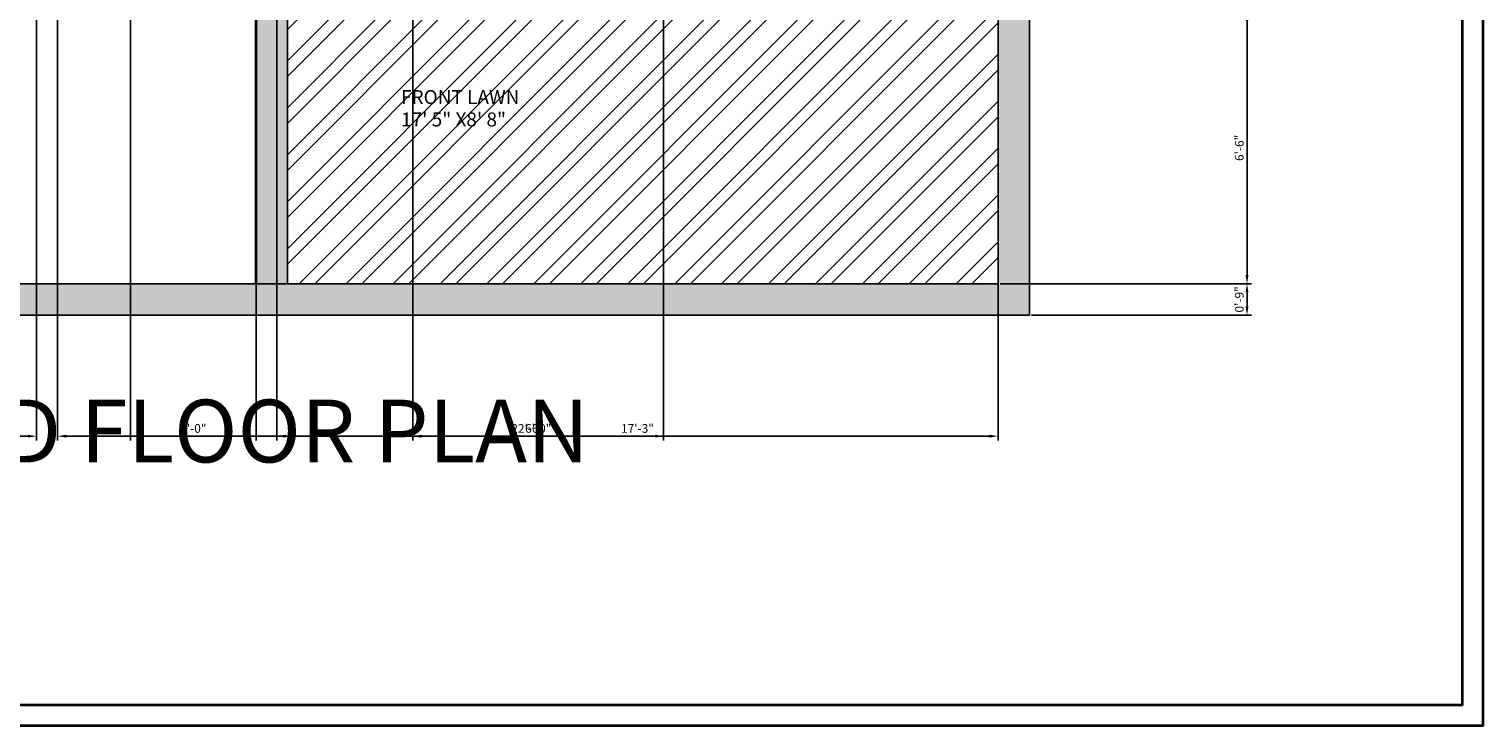
# Model space of a CAD drawing. Units: inches. Extents: x 2004 to 2661, y 1548 to 2351.
# Tile 2 of 5: x 2244 to 2661, y 1548 to 1748. Entities that reach past the tile are written whole.
import ezdxf

# ---------------------------------------------------------------- set-up
doc = ezdxf.new("R2010")
doc.units = ezdxf.units.IN
for name, color, linetype, lineweight in [('A-ANNO-DIMS', 2, 'Continuous', 18), ('A-ANNO-TEXT', 7, 'Continuous', 25), ('A-ANNO-TTLB', 7, 'Continuous', 35), ('A-AREA-IDEN', 7, 'Continuous', 18), ('A-WALL', 7, 'Continuous', 35), ('C-PROP', 7, 'Continuous', 25)]:
    doc.layers.add(name, color=color, linetype=linetype, lineweight=lineweight)
doc.layers.add('A-FLOR-PATT', color=18, linetype='Continuous', lineweight=13, true_color=0x000000)
doc.layers.add('A-WALL-PATT', color=18, linetype='Continuous', lineweight=13, true_color=0x000000)
doc.styles.get("Standard").update_dxf_attribs({"font": 'arial.ttf'})
doc.dimstyles.new('Copy of ISO-25', dxfattribs={"dimtxt": 2.5, "dimasz": 2.5, "dimexe": 1.25, "dimexo": 0.625, "dimtad": 1, "dimlunit": 4, "dimtxsty": 'Standard', "dimcen": 2.5, "dimadec": 0, "dimazin": 0, "dimtfac": 1, "dimtmove": 0, "dimatfit": 3, "dimfxl": 1, "dimarcsym": 0})

# ---------------------------------------------------------------- blocks, each defined once
blk = doc.blocks.new('*D37')
at = {"layer": 'A-ANNO-DIMS', "color": 0, "lineweight": -2, "transparency": 16777216}
for p, q in [((2246.26, 2082.47), (2246.26, 1630.09)), ((2144.26, 2046.47), (2144.26, 1630.09)), ((2146.76, 1631.34), (2243.76, 1631.34))]:
    blk.add_line(p, q, dxfattribs=at)
at = {"layer": 'A-ANNO-DIMS', "color": 0, "transparency": 16777216}
for points in [[(2146.76, 1631.76), (2146.76, 1630.93), (2144.26, 1631.34)], [(2243.76, 1631.76), (2243.76, 1630.93), (2246.26, 1631.34)]]:
    blk.add_solid(points, dxfattribs=at)
at = {"layer": 'Defpoints', "color": 0, "transparency": 16777216}
for p in [(2246.26, 2083.09), (2144.26, 2047.09), (2246.26, 1631.34)]:
    blk.add_point(p, dxfattribs=at)
at = {"layer": 'A-ANNO-DIMS', "color": 0, "transparency": 16777216, "insert": (2195.26, 1633.24), "char_height": 2.5, "attachment_point": 5}
blk.add_mtext('8\'-6"', dxfattribs=at)
blk = doc.blocks.new('*D39')
at = {"layer": 'A-ANNO-DIMS', "color": 0, "lineweight": -2, "transparency": 16777216}
for p, q in [((2252.26, 1887.47), (2252.26, 1630.09)), ((2522.26, 1887.47), (2522.26, 1630.09)), ((2254.76, 1631.34), (2519.76, 1631.34))]:
    blk.add_line(p, q, dxfattribs=at)
at = {"layer": 'A-ANNO-DIMS', "color": 0, "transparency": 16777216}
for points in [[(2254.76, 1631.76), (2254.76, 1630.93), (2252.26, 1631.34)], [(2519.76, 1631.76), (2519.76, 1630.93), (2522.26, 1631.34)]]:
    blk.add_solid(points, dxfattribs=at)
at = {"layer": 'Defpoints', "color": 0, "transparency": 16777216}
for p in [(2252.26, 1888.09), (2522.26, 1888.09), (2522.26, 1631.34)]:
    blk.add_point(p, dxfattribs=at)
at = {"layer": 'A-ANNO-DIMS', "color": 0, "transparency": 16777216, "insert": (2387.26, 1633.24), "char_height": 2.5, "attachment_point": 5}
blk.add_mtext('22\'-6"', dxfattribs=at)
blk = doc.blocks.new('*D40')
at = {"layer": 'A-ANNO-DIMS', "color": 0, "lineweight": -2, "transparency": 16777216}
for p, q in [((2522.88, 1753.09), (2594.98, 1753.09)), ((2593.73, 1750.59), (2593.73, 1677.59)), ((2522.88, 1675.09), (2594.98, 1675.09))]:
    blk.add_line(p, q, dxfattribs=at)
at = {"layer": 'A-ANNO-DIMS', "color": 0, "transparency": 16777216}
for points in [[(2593.31, 1750.59), (2594.15, 1750.59), (2593.73, 1753.09)], [(2593.31, 1677.59), (2594.15, 1677.59), (2593.73, 1675.09)]]:
    blk.add_solid(points, dxfattribs=at)
at = {"layer": 'Defpoints', "color": 0, "transparency": 16777216}
for p in [(2522.26, 1753.09), (2522.26, 1675.09), (2593.73, 1675.09)]:
    blk.add_point(p, dxfattribs=at)
at = {"layer": 'A-ANNO-DIMS', "color": 0, "transparency": 16777216, "insert": (2591.83, 1714.09), "char_height": 2.5, "attachment_point": 5, "rotation": 90}
blk.add_mtext('6\'-6"', dxfattribs=at)
blk = doc.blocks.new('*D41')
at = {"layer": 'A-ANNO-DIMS', "color": 0, "lineweight": -2, "transparency": 16777216}
for p, q in [((2318.26, 1675.72), (2318.26, 2346.91)), ((2320.76, 2345.66), (2519.76, 2345.66)), ((2522.26, 1675.72), (2522.26, 2346.91))]:
    blk.add_line(p, q, dxfattribs=at)
at = {"layer": 'A-ANNO-DIMS', "color": 0, "transparency": 16777216}
for points in [[(2320.76, 2346.07), (2320.76, 2345.24), (2318.26, 2345.66)], [(2519.76, 2346.07), (2519.76, 2345.24), (2522.26, 2345.66)]]:
    blk.add_solid(points, dxfattribs=at)
at = {"layer": 'Defpoints', "color": 0, "transparency": 16777216}
for p in [(2522.26, 2345.66), (2318.26, 1675.09), (2522.26, 1675.09)]:
    blk.add_point(p, dxfattribs=at)
at = {"layer": 'A-ANNO-DIMS', "color": 0, "transparency": 16777216, "insert": (2420.26, 2347.56), "char_height": 2.5, "attachment_point": 5}
blk.add_mtext('17\'-0"', dxfattribs=at)
blk = doc.blocks.new('*D42')
at = {"layer": 'A-ANNO-DIMS', "color": 0, "lineweight": -2, "transparency": 16777216}
for p, q in [((2315.26, 2256.47), (2315.26, 1630.09)), ((2522.26, 2256.47), (2522.26, 1630.09)), ((2317.76, 1631.34), (2519.76, 1631.34))]:
    blk.add_line(p, q, dxfattribs=at)
at = {"layer": 'A-ANNO-DIMS', "color": 0, "transparency": 16777216}
for points in [[(2317.76, 1631.76), (2317.76, 1630.93), (2315.26, 1631.34)], [(2519.76, 1631.76), (2519.76, 1630.93), (2522.26, 1631.34)]]:
    blk.add_solid(points, dxfattribs=at)
at = {"layer": 'Defpoints', "color": 0, "transparency": 16777216}
for p in [(2315.26, 2257.09), (2522.26, 2257.09), (2522.26, 1631.34)]:
    blk.add_point(p, dxfattribs=at)
at = {"layer": 'A-ANNO-DIMS', "color": 0, "transparency": 16777216, "insert": (2418.76, 1633.24), "char_height": 2.5, "attachment_point": 5}
blk.add_mtext('17\'-3"', dxfattribs=at)
blk = doc.blocks.new('*D43')
at = {"layer": 'A-ANNO-DIMS', "color": 0, "lineweight": -2, "transparency": 16777216}
for p, q in [((2522.88, 1675.09), (2594.98, 1675.09)), ((2593.73, 1668.59), (2593.73, 1672.59)), ((2531.88, 1666.09), (2594.98, 1666.09))]:
    blk.add_line(p, q, dxfattribs=at)
at = {"layer": 'A-ANNO-DIMS', "color": 0, "transparency": 16777216}
for points in [[(2593.31, 1672.59), (2594.15, 1672.59), (2593.73, 1675.09)], [(2593.31, 1668.59), (2594.15, 1668.59), (2593.73, 1666.09)]]:
    blk.add_solid(points, dxfattribs=at)
at = {"layer": 'Defpoints', "color": 0, "transparency": 16777216}
for p in [(2522.26, 1675.09), (2593.73, 1675.09), (2531.26, 1666.09)]:
    blk.add_point(p, dxfattribs=at)
at = {"layer": 'A-ANNO-DIMS', "color": 0, "transparency": 16777216, "insert": (2591.83, 1670.59), "char_height": 2.5, "attachment_point": 5, "rotation": 90}
blk.add_mtext('0\'-9"', dxfattribs=at)
blk = doc.blocks.new('*D45')
at = {"layer": 'A-ANNO-DIMS', "color": 0, "lineweight": -2, "transparency": 16777216}
for p, q in [((2273.26, 1878.47), (2273.26, 1630.09)), ((2309.26, 1878.47), (2309.26, 1630.09)), ((2275.76, 1631.34), (2306.76, 1631.34))]:
    blk.add_line(p, q, dxfattribs=at)
at = {"layer": 'A-ANNO-DIMS', "color": 0, "transparency": 16777216}
for points in [[(2275.76, 1631.76), (2275.76, 1630.93), (2273.26, 1631.34)], [(2306.76, 1631.76), (2306.76, 1630.93), (2309.26, 1631.34)]]:
    blk.add_solid(points, dxfattribs=at)
at = {"layer": 'Defpoints', "color": 0, "transparency": 16777216}
for p in [(2273.26, 1879.09), (2309.26, 1879.09), (2309.26, 1631.34)]:
    blk.add_point(p, dxfattribs=at)
at = {"layer": 'A-ANNO-DIMS', "color": 0, "transparency": 16777216, "insert": (2291.26, 1633.24), "char_height": 2.5, "attachment_point": 5}
blk.add_mtext('3\'-0"', dxfattribs=at)
blk = doc.blocks.new('*D47')
at = {"layer": 'A-ANNO-DIMS', "color": 0, "lineweight": -2, "transparency": 16777216}
for p, q in [((2354.26, 1881.47), (2354.26, 1630.09)), ((2426.26, 1881.47), (2426.26, 1630.09)), ((2356.76, 1631.34), (2423.76, 1631.34))]:
    blk.add_line(p, q, dxfattribs=at)
at = {"layer": 'A-ANNO-DIMS', "color": 0, "transparency": 16777216}
for points in [[(2356.76, 1631.76), (2356.76, 1630.93), (2354.26, 1631.34)], [(2423.76, 1631.76), (2423.76, 1630.93), (2426.26, 1631.34)]]:
    blk.add_solid(points, dxfattribs=at)
at = {"layer": 'Defpoints', "color": 0, "transparency": 16777216}
for p in [(2354.26, 1882.09), (2426.26, 1882.09), (2426.26, 1631.34)]:
    blk.add_point(p, dxfattribs=at)
at = {"layer": 'A-ANNO-DIMS', "color": 0, "transparency": 16777216, "insert": (2390.26, 1633.24), "char_height": 2.5, "attachment_point": 5}
blk.add_mtext('6\'-0"', dxfattribs=at)

msp = doc.modelspace()

# ---------------------------------------------------------------- hatches: boundary and pattern name
at = {"layer": 'A-FLOR-PATT'}
h = msp.add_hatch(dxfattribs=at)
h.set_pattern_fill('ANSI32', color=256)
h.paths.add_polyline_path([(2522.257, 2257.093), (2466.833, 2257.093), (2315.257, 2257.093), (2418.757, 2233.093)])
h.paths.add_polyline_path([(2418.757, 2233.093), (2315.257, 2257.093), (2315.257, 2209.093)])
h.paths.add_polyline_path([(2418.757, 2233.093), (2315.257, 2209.093), (2522.257, 2209.093)])
h.paths.add_polyline_path([(2522.257, 2257.093), (2418.757, 2233.093), (2522.257, 2209.093)])
h.paths.add_polyline_path([(2522.257, 1753.093), (2318.257, 1753.093), (2318.257, 1675.093), (2522.257, 1675.093)])
h.paths.add_polyline_path([(2210.267, 2081.517), (2210.233, 2081.517), (2210.233, 2083.093), (2246.257, 2083.093), (2246.257, 2119.093), (2144.257, 2119.093), (2144.257, 2047.093), (2244.938, 2047.093, -0.390864)])
h.paths.add_polyline_path([(2171.613, 2077.721), (2161.069, 2080.96), (2161.193, 2075.729), (2163.808, 2075.791), (2163.932, 2070.56), (2162.189, 2070.519), (2162.106, 2074.006), (2161.234, 2073.986), (2161.338, 2069.627), (2147.389, 2069.296), (2146.521, 2105.911), (2160.469, 2106.241), (2160.738, 2094.908), (2171.117, 2098.643, -0.7025712), (2195.775, 2088.761, -0.7025621)], flags=16)
h.paths.add_polyline_path([(2171.53, 2081.208), (2171.2, 2095.156, -0.7345333), (2194.031, 2088.72, -0.7345297)], flags=0)
h.paths.add_polyline_path([(2158.245, 2071.298), (2150.835, 2071.122, -0.4142136), (2149.061, 2072.388), (2148.347, 2102.465, -0.4142136), (2149.614, 2104.239), (2157.024, 2104.415, -0.4142136), (2158.798, 2103.149), (2159.512, 2073.072, -0.4142136)], flags=0)
h.paths.add_polyline_path([(2522.257, 2200.093), (2517.397, 2200.093), (2517.397, 2185.232), (2505.384, 2185.232), (2509.08, 2174.143, -0.7025712), (2497.991, 2148.268, -0.7025621), (2486.902, 2174.142), (2490.599, 2185.232), (2485.054, 2185.232), (2485.054, 2182.459), (2479.509, 2182.459), (2479.509, 2184.307), (2483.206, 2184.307), (2483.206, 2185.232), (2478.585, 2185.232), (2478.585, 2200.093), (2459.257, 2200.093), (2459.257, 2106.686, -0.3761573), (2493.676, 2139.619), (2493.676, 2139.653), (2495.257, 2139.653), (2495.257, 2104.093), (2522.257, 2104.093)])
h.paths.add_polyline_path([(2349.854, 1719.146), (2381.921, 1719.146), (2381.921, 1725.273), (2349.854, 1725.273)], flags=24)
h.paths.add_polyline_path([(2349.84, 1725.558), (2388.851, 1725.558), (2388.851, 1731.767), (2349.84, 1731.767)], flags=24)
h.paths.add_polyline_path([(2152.908, 2086.679), (2181.867, 2086.679), (2181.867, 2092.806), (2152.908, 2092.806)], flags=8)
h.paths.add_polyline_path([(2152.895, 2093.091), (2174.525, 2093.091), (2174.525, 2099.3), (2152.895, 2099.3)], flags=8)
h.paths.add_polyline_path([(2515.001, 2150.174), (2515.001, 2154.033), (2509.85, 2154.033), (2509.85, 2150.174)], flags=24)
h.paths.add_polyline_path([(2469.272, 2171.563), (2498.231, 2171.563), (2498.231, 2177.69), (2469.272, 2177.69)], flags=24)
h.paths.add_polyline_path([(2469.258, 2177.975), (2490.888, 2177.975), (2490.888, 2184.184), (2469.258, 2184.184)], flags=24)
at = {"layer": 'A-WALL-PATT'}
h = msp.add_hatch(color=256, dxfattribs=at)
h.dxf.hatch_style = 1
h.paths.add_polyline_path([(2315.257, 2266.093), (2135.257, 2266.093), (2135.257, 1666.093), (2531.257, 1666.093), (2531.257, 1753.093), (2522.257, 1753.093), (2522.257, 1675.093), (2144.257, 1675.093), (2144.257, 2038.093), (2180.257, 2038.093), (2180.257, 2047.093), (2144.257, 2047.093), (2144.257, 2257.093), (2309.257, 2257.093), (2315.257, 2257.093)])
h.paths.add_polyline_path([(2522.257, 2266.093), (2315.257, 2266.093), (2315.257, 2257.093), (2522.257, 2257.093)], flags=17)
h.paths.add_polyline_path([(2368.773, 2209.093), (2315.257, 2209.093), (2309.257, 2209.093), (2309.257, 2119.093), (2309.257, 2083.093), (2315.257, 2083.093), (2315.257, 2119.093), (2315.257, 2200.093), (2368.773, 2200.093)], flags=17)
h.paths.add_polyline_path([(2459.257, 2209.093), (2428.773, 2209.093), (2428.773, 2200.093), (2453.257, 2200.093), (2459.257, 2200.093)], flags=17)
h.paths.add_polyline_path([(2522.257, 2209.093), (2483.257, 2209.093), (2483.257, 2200.093), (2522.257, 2200.093)], flags=17)
h.paths.add_polyline_path([(2522.257, 2044.093), (2459.257, 2044.093), (2459.257, 2056.073, -0.004139), (2458.66, 2056.069), (2453.257, 2056.069), (2453.257, 2044.093), (2315.257, 2044.093), (2315.257, 2046.941, -0.0039864), (2314.68, 2046.936), (2309.257, 2046.936), (2309.257, 2038.093), (2315.257, 2038.093), (2522.257, 2038.093)], flags=17)
h.paths.add_polyline_path([(2531.257, 2266.093), (2522.257, 2266.093), (2522.257, 2257.093), (2522.257, 2209.093), (2522.257, 2200.093), (2522.257, 2104.093), (2522.257, 1762.093), (2498.257, 1762.093), (2498.257, 1753.093), (2522.257, 1753.093), (2531.257, 1753.093)], flags=17)
h.paths.add_polyline_path([(2522.257, 2104.093), (2495.257, 2104.093), (2495.257, 2103.514), (2495.257, 2098.093), (2503.401, 2098.093), (2522.257, 2098.093)], flags=17)
h.paths.add_polyline_path([(2455.748, 2073.874), (2484.708, 2073.874), (2484.708, 2080.001), (2455.748, 2080.001)], flags=25)
h.paths.add_polyline_path([(2455.735, 2080.287), (2477.056, 2080.287), (2477.056, 2086.492), (2455.735, 2086.492)], flags=25)
h.paths.add_polyline_path([(2469.272, 2171.563), (2498.231, 2171.563), (2498.231, 2177.69), (2469.272, 2177.69)], flags=25)
h.paths.add_polyline_path([(2469.258, 2177.975), (2490.888, 2177.975), (2490.888, 2184.184), (2469.258, 2184.184)], flags=25)
h.paths.add_polyline_path([(2360.849, 2078.511), (2396.023, 2078.511), (2396.023, 2084.638), (2360.849, 2084.638)], flags=25)
h.paths.add_polyline_path([(2360.835, 2084.923), (2394.883, 2084.923), (2394.883, 2091.132), (2360.835, 2091.132)], flags=25)
h = msp.add_hatch(color=256, dxfattribs=at)
h.dxf.hatch_style = 1
h.paths.add_polyline_path([(2252.257, 2038.093), (2252.257, 2047.093), (2246.257, 2047.093), (2204.257, 2047.093), (2204.257, 2038.093), (2243.257, 2038.093), (2243.257, 1888.093), (2243.257, 1879.093), (2273.257, 1879.093), (2273.257, 1888.093), (2252.257, 1888.093)])
h.paths.add_polyline_path([(2273.257, 2125.093), (2144.257, 2125.093), (2144.257, 2119.093), (2246.257, 2119.093), (2273.257, 2119.093)])
h.paths.add_polyline_path([(2459.257, 2200.093), (2453.257, 2200.093), (2453.257, 2092.093), (2459.257, 2092.093)])
h.paths.add_polyline_path([(2522.257, 1888.093), (2426.257, 1888.093), (2426.257, 1882.093), (2522.257, 1882.093)])
h.paths.add_polyline_path([(2460.257, 1834.093), (2454.257, 1834.093), (2454.257, 1762.093), (2460.257, 1762.093)])
h.paths.add_polyline_path([(2460.257, 1882.093), (2454.257, 1882.093), (2454.257, 1870.093), (2460.257, 1870.093)])
h.paths.add_polyline_path([(2462.257, 1762.093), (2460.257, 1762.093), (2454.257, 1762.093), (2390.257, 1762.093), (2390.257, 1753.093), (2462.257, 1753.093)])
h.paths.add_polyline_path([(2342.257, 1762.093), (2318.257, 1762.093), (2318.257, 1882.093), (2318.257, 1888.093), (2309.257, 1888.093), (2309.257, 1879.093), (2309.257, 1753.093), (2318.257, 1753.093), (2342.257, 1753.093)])
h.paths.add_polyline_path([(2354.257, 1888.093), (2318.257, 1888.093), (2318.257, 1882.093), (2354.257, 1882.093)])
h.paths.add_polyline_path([(2318.257, 1753.093), (2309.257, 1753.093), (2309.257, 1675.093), (2318.257, 1675.093)])
h.paths.add_polyline_path([(2207.257, 1884.43), (2207.257, 1888.093), (2183.257, 1888.093), (2183.257, 1879.093), (2207.257, 1879.093)])
h.paths.add_polyline_path([(2252.257, 2119.093), (2246.257, 2119.093), (2246.257, 2083.093), (2251.66, 2083.093), (2252.257, 2083.093)])
h.paths.add_polyline_path([(2315.257, 2257.093), (2309.257, 2257.093), (2309.257, 2209.093), (2315.257, 2209.093)])

# ---------------------------------------------------------------- linework, layer by layer
at = {"layer": 'A-ANNO-TTLB'}
for points in [[(2014.058, 2344.754), (2661.447, 2344.754), (2661.447, 1548.19), (2014.058, 1548.19)], [(2020.058, 2338.754), (2655.447, 2338.754), (2655.447, 1554.19), (2020.058, 1554.19)]]:
    msp.add_lwpolyline(points, close=True, dxfattribs=at)
at = {"layer": 'A-WALL'}
msp.add_line((2309.257, 1675.093), (2309.257, 1879.093), dxfattribs=at)
at = {"layer": 'C-PROP'}
for p, q in [((2531.257, 2266.093), (2531.257, 1666.093)), ((2318.257, 1753.093), (2318.257, 1675.093)), ((2522.257, 1753.093), (2522.257, 1675.093)), ((2522.257, 1675.093), (2144.257, 1675.093)), ((2144.257, 1675.093), (2309.257, 1675.093)), ((2531.257, 1666.093), (2135.257, 1666.093))]:
    msp.add_line(p, q, dxfattribs=at)

# ---------------------------------------------------------------- texts
at = {"layer": 'A-ANNO-TEXT'}
msp.add_text('GROUND FLOOR PLAN', height=18, dxfattribs=at).set_placement((2150.24, 1623.82))
at = {"layer": 'A-AREA-IDEN'}
for s, p in [('FRONT LAWN', (2350.875, 1726.661)), ('17\' 5" X8\' 8"', (2350.875, 1720.235))]:
    msp.add_text(s, height=4, dxfattribs=at).set_placement(p)

# ---------------------------------------------------------------- dimensions: what is measured, and where the dimension line sits
at = {"layer": 'A-ANNO-DIMS'}
for base, p1, p2, picture, middle in [((2522.257, 2345.658), (2318.257, 1675.093), (2522.257, 1675.093), '*D41', (2420.257, 2347.559)), ((2522.257, 1631.343), (2315.257, 2257.093), (2522.257, 2257.093), '*D42', (2418.757, 1633.245)), ((2246.257, 1631.343), (2144.257, 2047.093), (2246.257, 2083.093), '*D37', (2195.257, 1633.244)), ((2522.257, 1631.343), (2252.257, 1888.093), (2522.257, 1888.093), '*D39', (2387.257, 1633.244)), ((2309.257, 1631.343), (2273.257, 1879.093), (2309.257, 1879.093), '*D45', (2291.257, 1633.245)), ((2426.257, 1631.343), (2354.257, 1882.093), (2426.257, 1882.093), '*D47', (2390.257, 1633.244))]:
    dim = msp.add_linear_dim(base=base, p1=p1, p2=p2, dimstyle='Copy of ISO-25', override={"dimdec": 1, "dimlfac": 1, "dimrnd": 0, "dimzin": 1, "dimdsep": 46, "dimlunit": 4, "dimfrac": 2}, dxfattribs=at)
    dim.commit()
    dim.dimension.update_dxf_attribs({"geometry": picture, "text_midpoint": middle})
for p1, picture, middle in [((2522.257, 1753.093), '*D40', (2591.83, 1714.093)), ((2531.257, 1666.093), '*D43', (2591.83, 1670.593))]:
    dim = msp.add_linear_dim(base=(2593.731, 1675.093), p1=p1, p2=(2522.257, 1675.093), angle=90, dimstyle='Copy of ISO-25', override={"dimdec": 1, "dimlfac": 1, "dimrnd": 0, "dimzin": 1, "dimdsep": 46, "dimlunit": 4, "dimfrac": 2}, dxfattribs=at)
    dim.commit()
    dim.dimension.update_dxf_attribs({"geometry": picture, "text_midpoint": middle})

doc.saveas('drawing.dxf')
